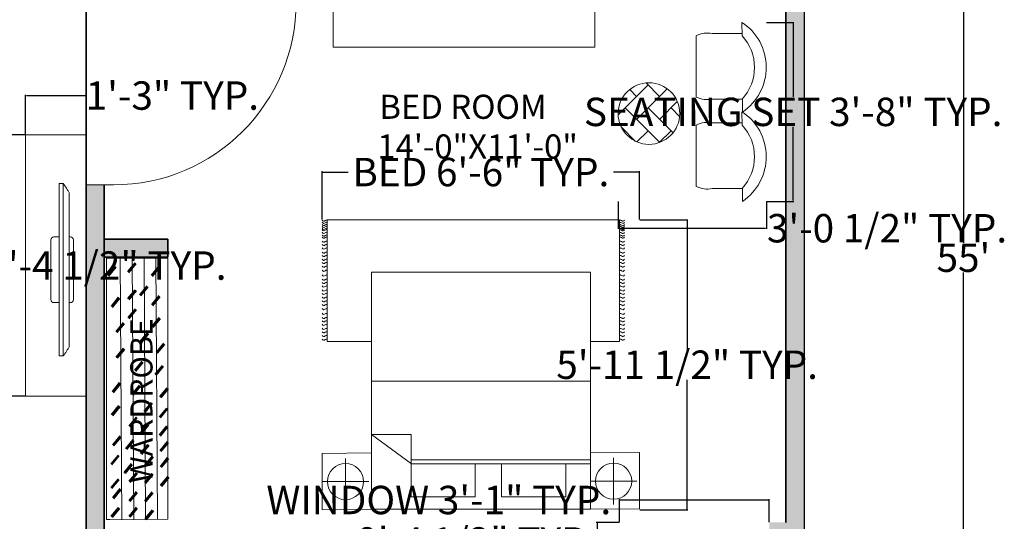
# Model space of a CAD drawing. Units: inches. Extents: x 0 to 4258, y 0 to 3769.
# Tile 25 of 30: x 3845 to 4088, y 3261 to 3385. Entities that reach past the tile are written whole.
import ezdxf

# ---------------------------------------------------------------- set-up
doc = ezdxf.new("R2010")
doc.units = ezdxf.units.IN
doc.header["$MEASUREMENT"] = 0
doc.layers.get('0').update_dxf_attribs({"color": 16})
for name, color, linetype, lineweight in [('A-ANNO-DIMS', 250, 'Continuous', 18), ('A-ANNO-TEXT', 250, 'Continuous', 18), ('A-AREA-IDEN', 250, 'Continuous', 18), ('A-CASE', 150, 'Continuous', 18), ('A-CASE-PATT', 251, 'Continuous', 13), ('A-EQPM', 8, 'Continuous', 18), ('A-WALL-PATT', 16, 'Continuous', 13), ('C-PROP', 150, 'Continuous', 25), ('doors', 250, 'Continuous', 18), ('furniture', 13, 'Continuous', 18), ('walls', 251, 'Continuous', 35)]:
    doc.layers.add(name, color=color, linetype=linetype, lineweight=lineweight)
doc.styles.get("Standard").update_dxf_attribs({"font": 'arial.ttf'})
doc.dimstyles.get("Standard").update_dxf_attribs({"dimtxt": 7, "dimasz": 0.18, "dimexe": 0.18, "dimexo": 0.0625, "dimgap": 0.09, "dimtad": 0, "dimtih": 1, "dimtoh": 1, "dimzin": 0, "dimdsep": 46, "dimlunit": 3, "dimtxsty": 'Standard', "dimcen": 0.09, "dimadec": 0, "dimazin": 0, "dimtfac": 1, "dimtofl": 0, "dimtmove": 0, "dimatfit": 3, "dimfxl": 1, "dimtolj": 1, "dimtzin": 0, "dimarcsym": 0})

# ---------------------------------------------------------------- blocks, each defined once
blk = doc.blocks.new('PLASMA-LARGE')
at = {"layer": 'furniture'}
for p, q in [((-7.26, 0), (7.26, 0)), ((-18.61, -1), (18.61, -1)), ((-8, -1), (-8, -0.74)), ((8, -1), (8, -0.74)), ((-21, -2.5), (21, -2.5)), ((-21, -2.5), (-21, -3.5)), ((-21, -3.5), (21, -3.5)), ((-8, -3.5), (-8, -4.76)), ((8, -3.5), (8, -4.76)), ((21, -2.5), (21, -3.5)), ((-7.26, -5.5), (7.26, -5.5))]:
    blk.add_line(p, q, dxfattribs=at)
for centre, radius, start, end in [((-7.26, -0.74), 0.744, 90, 180), ((7.26, -0.74), 0.744, 0, 90), ((-13.97, -11.05), 11.07, 114.7602, 129.4175), ((13.97, -11.05), 11.07, 50.5825, 65.2398), ((-7.26, -4.76), 0.744, 180, 270), ((7.26, -4.76), 0.744, 270, 0)]:
    blk.add_arc(centre, radius, start, end, dxfattribs=at)
blk = doc.blocks.new('CARPET')
at = {"layer": 'furniture'}
for p, q in [((-51.53, -98.11), (-51.53, -55.12)), ((-51.53, -55.12), (-41.27, -55.12)), ((36, -55.12), (51.55, -55.12)), ((51.55, -55.12), (51.55, -98.11)), ((51.55, -98.11), (-51.53, -98.11))]:
    blk.add_line(p, q, dxfattribs=at)
for points, knots in [([(-53.37, -55.99), (-53.22, -55.8), (-52.9, -55.41), (-52.34, -55.8), (-51.89, -56.08), (-51.65, -55.91), (-51.53, -55.83)], [0, 0, 0, 0, 0.653278, 1.290138, 1.740457, 2.114451, 2.114451, 2.114451, 2.114451]), ([(53.37, -55.99), (53.22, -55.8), (52.9, -55.41), (52.34, -55.8), (51.89, -56.08), (51.65, -55.91), (51.53, -55.83)], [0, 0, 0, 0, 0.653278, 1.290138, 1.740457, 2.114451, 2.114451, 2.114451, 2.114451]), ([(-53.37, -57.26), (-53.22, -57.07), (-52.9, -56.67), (-52.34, -57.07), (-51.89, -57.35), (-51.65, -57.17), (-51.53, -57.1)], [0, 0, 0, 0, 0.653278, 1.290138, 1.740457, 2.114451, 2.114451, 2.114451, 2.114451]), ([(-53.37, -58.59), (-53.22, -58.4), (-52.9, -58.01), (-52.34, -58.4), (-51.89, -58.68), (-51.65, -58.5), (-51.53, -58.43)], [0, 0, 0, 0, 0.653278, 1.290138, 1.740457, 2.114451, 2.114451, 2.114451, 2.114451]), ([(53.37, -57.26), (53.22, -57.07), (52.9, -56.67), (52.34, -57.07), (51.89, -57.35), (51.65, -57.17), (51.53, -57.1)], [0, 0, 0, 0, 0.653278, 1.290138, 1.740457, 2.114451, 2.114451, 2.114451, 2.114451]), ([(53.37, -58.59), (53.22, -58.4), (52.9, -58.01), (52.34, -58.4), (51.89, -58.68), (51.65, -58.5), (51.53, -58.43)], [0, 0, 0, 0, 0.653278, 1.290138, 1.740457, 2.114451, 2.114451, 2.114451, 2.114451]), ([(-53.37, -59.78), (-53.22, -59.58), (-52.9, -59.19), (-52.34, -59.58), (-51.89, -59.86), (-51.65, -59.69), (-51.53, -59.61)], [0, 0, 0, 0, 0.653278, 1.290138, 1.740457, 2.114451, 2.114451, 2.114451, 2.114451]), ([(-53.37, -61.22), (-53.22, -61.02), (-52.9, -60.63), (-52.34, -61.02), (-51.89, -61.3), (-51.65, -61.13), (-51.53, -61.05)], [0, 0, 0, 0, 0.653278, 1.290138, 1.740457, 2.114451, 2.114451, 2.114451, 2.114451]), ([(-53.37, -62.44), (-53.22, -62.25), (-52.9, -61.86), (-52.34, -62.25), (-51.89, -62.53), (-51.65, -62.36), (-51.53, -62.28)], [0, 0, 0, 0, 0.653278, 1.290138, 1.740457, 2.114451, 2.114451, 2.114451, 2.114451]), ([(53.37, -59.78), (53.22, -59.58), (52.9, -59.19), (52.34, -59.58), (51.89, -59.86), (51.65, -59.69), (51.53, -59.61)], [0, 0, 0, 0, 0.653278, 1.290138, 1.740457, 2.114451, 2.114451, 2.114451, 2.114451]), ([(53.37, -61.22), (53.22, -61.02), (52.9, -60.63), (52.34, -61.02), (51.89, -61.3), (51.65, -61.13), (51.53, -61.05)], [0, 0, 0, 0, 0.653278, 1.290138, 1.740457, 2.114451, 2.114451, 2.114451, 2.114451]), ([(53.37, -62.44), (53.22, -62.25), (52.9, -61.86), (52.34, -62.25), (51.89, -62.53), (51.65, -62.36), (51.53, -62.28)], [0, 0, 0, 0, 0.653278, 1.290138, 1.740457, 2.114451, 2.114451, 2.114451, 2.114451]), ([(-53.37, -63.63), (-53.22, -63.43), (-52.9, -63.04), (-52.34, -63.43), (-51.89, -63.72), (-51.65, -63.54), (-51.53, -63.46)], [0, 0, 0, 0, 0.653278, 1.290138, 1.740457, 2.114451, 2.114451, 2.114451, 2.114451]), ([(-53.37, -65.07), (-53.22, -64.87), (-52.9, -64.48), (-52.34, -64.87), (-51.89, -65.15), (-51.65, -64.98), (-51.53, -64.9)], [0, 0, 0, 0, 0.653278, 1.290138, 1.740457, 2.114451, 2.114451, 2.114451, 2.114451]), ([(53.37, -63.63), (53.22, -63.43), (52.9, -63.04), (52.34, -63.43), (51.89, -63.72), (51.65, -63.54), (51.53, -63.46)], [0, 0, 0, 0, 0.653278, 1.290138, 1.740457, 2.114451, 2.114451, 2.114451, 2.114451]), ([(53.37, -65.07), (53.22, -64.87), (52.9, -64.48), (52.34, -64.87), (51.89, -65.15), (51.65, -64.98), (51.53, -64.9)], [0, 0, 0, 0, 0.653278, 1.290138, 1.740457, 2.114451, 2.114451, 2.114451, 2.114451]), ([(-53.37, -66.76), (-53.22, -66.56), (-52.9, -66.17), (-52.34, -66.56), (-51.89, -66.84), (-51.65, -66.67), (-51.53, -66.59)], [0, 0, 0, 0, 0.653278, 1.290138, 1.740457, 2.114451, 2.114451, 2.114451, 2.114451]), ([(-53.37, -68.2), (-53.22, -68), (-52.9, -67.61), (-52.34, -68), (-51.89, -68.28), (-51.65, -68.11), (-51.53, -68.03)], [0, 0, 0, 0, 0.653278, 1.290138, 1.740457, 2.114451, 2.114451, 2.114451, 2.114451]), ([(-53.37, -69.53), (-53.22, -69.33), (-52.9, -68.94), (-52.34, -69.33), (-51.89, -69.61), (-51.65, -69.44), (-51.53, -69.36)], [0, 0, 0, 0, 0.653278, 1.290138, 1.740457, 2.114451, 2.114451, 2.114451, 2.114451]), ([(53.37, -66.76), (53.22, -66.56), (52.9, -66.17), (52.34, -66.56), (51.89, -66.84), (51.65, -66.67), (51.53, -66.59)], [0, 0, 0, 0, 0.653278, 1.290138, 1.740457, 2.114451, 2.114451, 2.114451, 2.114451]), ([(53.37, -68.2), (53.22, -68), (52.9, -67.61), (52.34, -68), (51.89, -68.28), (51.65, -68.11), (51.53, -68.03)], [0, 0, 0, 0, 0.653278, 1.290138, 1.740457, 2.114451, 2.114451, 2.114451, 2.114451]), ([(53.37, -69.53), (53.22, -69.33), (52.9, -68.94), (52.34, -69.33), (51.89, -69.61), (51.65, -69.44), (51.53, -69.36)], [0, 0, 0, 0, 0.653278, 1.290138, 1.740457, 2.114451, 2.114451, 2.114451, 2.114451]), ([(-53.37, -70.79), (-53.22, -70.6), (-52.9, -70.21), (-52.34, -70.6), (-51.89, -70.88), (-51.65, -70.7), (-51.53, -70.63)], [0, 0, 0, 0, 0.653278, 1.290138, 1.740457, 2.114451, 2.114451, 2.114451, 2.114451]), ([(-53.37, -72.12), (-53.22, -71.93), (-52.9, -71.54), (-52.34, -71.93), (-51.89, -72.21), (-51.65, -72.04), (-51.53, -71.96)], [0, 0, 0, 0, 0.653278, 1.290138, 1.740457, 2.114451, 2.114451, 2.114451, 2.114451]), ([(-53.37, -73.31), (-53.22, -73.11), (-52.9, -72.72), (-52.34, -73.11), (-51.89, -73.4), (-51.65, -73.22), (-51.53, -73.14)], [0, 0, 0, 0, 0.653278, 1.290138, 1.740457, 2.114451, 2.114451, 2.114451, 2.114451]), ([(53.37, -70.79), (53.22, -70.6), (52.9, -70.21), (52.34, -70.6), (51.89, -70.88), (51.65, -70.7), (51.53, -70.63)], [0, 0, 0, 0, 0.653278, 1.290138, 1.740457, 2.114451, 2.114451, 2.114451, 2.114451]), ([(53.37, -72.12), (53.22, -71.93), (52.9, -71.54), (52.34, -71.93), (51.89, -72.21), (51.65, -72.04), (51.53, -71.96)], [0, 0, 0, 0, 0.653278, 1.290138, 1.740457, 2.114451, 2.114451, 2.114451, 2.114451]), ([(53.37, -73.31), (53.22, -73.11), (52.9, -72.72), (52.34, -73.11), (51.89, -73.4), (51.65, -73.22), (51.53, -73.14)], [0, 0, 0, 0, 0.653278, 1.290138, 1.740457, 2.114451, 2.114451, 2.114451, 2.114451]), ([(-53.37, -74.75), (-53.22, -74.55), (-52.9, -74.16), (-52.34, -74.55), (-51.89, -74.83), (-51.65, -74.66), (-51.53, -74.58)], [0, 0, 0, 0, 0.653278, 1.290138, 1.740457, 2.114451, 2.114451, 2.114451, 2.114451]), ([(-53.37, -75.98), (-53.22, -75.78), (-52.9, -75.39), (-52.34, -75.78), (-51.89, -76.06), (-51.65, -75.89), (-51.53, -75.81)], [0, 0, 0, 0, 0.653278, 1.290138, 1.740457, 2.114451, 2.114451, 2.114451, 2.114451]), ([(53.37, -74.75), (53.22, -74.55), (52.9, -74.16), (52.34, -74.55), (51.89, -74.83), (51.65, -74.66), (51.53, -74.58)], [0, 0, 0, 0, 0.653278, 1.290138, 1.740457, 2.114451, 2.114451, 2.114451, 2.114451]), ([(53.37, -75.98), (53.22, -75.78), (52.9, -75.39), (52.34, -75.78), (51.89, -76.06), (51.65, -75.89), (51.53, -75.81)], [0, 0, 0, 0, 0.653278, 1.290138, 1.740457, 2.114451, 2.114451, 2.114451, 2.114451]), ([(-53.37, -77.16), (-53.22, -76.96), (-52.9, -76.57), (-52.34, -76.96), (-51.89, -77.25), (-51.65, -77.07), (-51.53, -76.99)], [0, 0, 0, 0, 0.653278, 1.290138, 1.740457, 2.114451, 2.114451, 2.114451, 2.114451]), ([(-53.37, -78.6), (-53.22, -78.4), (-52.9, -78.01), (-52.34, -78.4), (-51.89, -78.68), (-51.65, -78.51), (-51.53, -78.43)], [0, 0, 0, 0, 0.653278, 1.290138, 1.740457, 2.114451, 2.114451, 2.114451, 2.114451]), ([(-53.37, -80.29), (-53.22, -80.09), (-52.9, -79.7), (-52.34, -80.09), (-51.89, -80.37), (-51.65, -80.2), (-51.53, -80.12)], [0, 0, 0, 0, 0.653278, 1.290138, 1.740457, 2.114451, 2.114451, 2.114451, 2.114451]), ([(53.37, -77.16), (53.22, -76.96), (52.9, -76.57), (52.34, -76.96), (51.89, -77.25), (51.65, -77.07), (51.53, -76.99)], [0, 0, 0, 0, 0.653278, 1.290138, 1.740457, 2.114451, 2.114451, 2.114451, 2.114451]), ([(53.37, -78.6), (53.22, -78.4), (52.9, -78.01), (52.34, -78.4), (51.89, -78.68), (51.65, -78.51), (51.53, -78.43)], [0, 0, 0, 0, 0.653278, 1.290138, 1.740457, 2.114451, 2.114451, 2.114451, 2.114451]), ([(53.37, -80.29), (53.22, -80.09), (52.9, -79.7), (52.34, -80.09), (51.89, -80.37), (51.65, -80.2), (51.53, -80.12)], [0, 0, 0, 0, 0.653278, 1.290138, 1.740457, 2.114451, 2.114451, 2.114451, 2.114451]), ([(-53.37, -81.73), (-53.22, -81.53), (-52.9, -81.14), (-52.34, -81.53), (-51.89, -81.81), (-51.65, -81.64), (-51.53, -81.56)], [0, 0, 0, 0, 0.653278, 1.290138, 1.740457, 2.114451, 2.114451, 2.114451, 2.114451]), ([(-53.37, -83.06), (-53.22, -82.86), (-52.9, -82.47), (-52.34, -82.86), (-51.89, -83.14), (-51.65, -82.97), (-51.53, -82.89)], [0, 0, 0, 0, 0.653278, 1.290138, 1.740457, 2.114451, 2.114451, 2.114451, 2.114451]), ([(53.37, -81.73), (53.22, -81.53), (52.9, -81.14), (52.34, -81.53), (51.89, -81.81), (51.65, -81.64), (51.53, -81.56)], [0, 0, 0, 0, 0.653278, 1.290138, 1.740457, 2.114451, 2.114451, 2.114451, 2.114451]), ([(53.37, -83.06), (53.22, -82.86), (52.9, -82.47), (52.34, -82.86), (51.89, -83.14), (51.65, -82.97), (51.53, -82.89)], [0, 0, 0, 0, 0.653278, 1.290138, 1.740457, 2.114451, 2.114451, 2.114451, 2.114451]), ([(-53.37, -84.18), (-53.22, -83.99), (-52.9, -83.6), (-52.34, -83.99), (-51.89, -84.27), (-51.65, -84.09), (-51.53, -84.02)], [0, 0, 0, 0, 0.653278, 1.290138, 1.740457, 2.114451, 2.114451, 2.114451, 2.114451]), ([(-53.37, -85.51), (-53.22, -85.32), (-52.9, -84.93), (-52.34, -85.32), (-51.89, -85.6), (-51.65, -85.42), (-51.53, -85.35)], [0, 0, 0, 0, 0.653278, 1.290138, 1.740457, 2.114451, 2.114451, 2.114451, 2.114451]), ([(-53.37, -86.7), (-53.22, -86.5), (-52.9, -86.11), (-52.34, -86.5), (-51.89, -86.78), (-51.65, -86.61), (-51.53, -86.53)], [0, 0, 0, 0, 0.653278, 1.290138, 1.740457, 2.114451, 2.114451, 2.114451, 2.114451]), ([(53.37, -84.18), (53.22, -83.99), (52.9, -83.6), (52.34, -83.99), (51.89, -84.27), (51.65, -84.09), (51.53, -84.02)], [0, 0, 0, 0, 0.653278, 1.290138, 1.740457, 2.114451, 2.114451, 2.114451, 2.114451]), ([(53.37, -85.51), (53.22, -85.32), (52.9, -84.93), (52.34, -85.32), (51.89, -85.6), (51.65, -85.42), (51.53, -85.35)], [0, 0, 0, 0, 0.653278, 1.290138, 1.740457, 2.114451, 2.114451, 2.114451, 2.114451]), ([(53.37, -86.7), (53.22, -86.5), (52.9, -86.11), (52.34, -86.5), (51.89, -86.78), (51.65, -86.61), (51.53, -86.53)], [0, 0, 0, 0, 0.653278, 1.290138, 1.740457, 2.114451, 2.114451, 2.114451, 2.114451]), ([(-53.37, -88.14), (-53.22, -87.94), (-52.9, -87.55), (-52.34, -87.94), (-51.89, -88.22), (-51.65, -88.05), (-51.53, -87.97)], [0, 0, 0, 0, 0.653278, 1.290138, 1.740457, 2.114451, 2.114451, 2.114451, 2.114451]), ([(-53.37, -89.36), (-53.22, -89.17), (-52.9, -88.78), (-52.34, -89.17), (-51.89, -89.45), (-51.65, -89.28), (-51.53, -89.2)], [0, 0, 0, 0, 0.653278, 1.290138, 1.740457, 2.114451, 2.114451, 2.114451, 2.114451]), ([(-53.37, -90.55), (-53.22, -90.35), (-52.9, -89.96), (-52.34, -90.35), (-51.89, -90.64), (-51.65, -90.46), (-51.53, -90.38)], [0, 0, 0, 0, 0.653278, 1.290138, 1.740457, 2.114451, 2.114451, 2.114451, 2.114451]), ([(53.37, -88.14), (53.22, -87.94), (52.9, -87.55), (52.34, -87.94), (51.89, -88.22), (51.65, -88.05), (51.53, -87.97)], [0, 0, 0, 0, 0.653278, 1.290138, 1.740457, 2.114451, 2.114451, 2.114451, 2.114451]), ([(53.37, -89.36), (53.22, -89.17), (52.9, -88.78), (52.34, -89.17), (51.89, -89.45), (51.65, -89.28), (51.53, -89.2)], [0, 0, 0, 0, 0.653278, 1.290138, 1.740457, 2.114451, 2.114451, 2.114451, 2.114451]), ([(53.37, -90.55), (53.22, -90.35), (52.9, -89.96), (52.34, -90.35), (51.9, -90.63), (51.66, -90.47), (51.55, -90.4)], [0, 0, 0, 0, 0.653278, 1.290138, 1.740457, 2.0926, 2.0926, 2.0926, 2.0926]), ([(-53.37, -91.99), (-53.22, -91.79), (-52.9, -91.4), (-52.34, -91.79), (-51.89, -92.07), (-51.65, -91.9), (-51.53, -91.82)], [0, 0, 0, 0, 0.653278, 1.290138, 1.740457, 2.114451, 2.114451, 2.114451, 2.114451]), ([(-53.37, -92.69), (-53.22, -92.48), (-52.9, -92.08), (-52.35, -92.49), (-51.89, -92.77), (-51.65, -92.6), (-51.53, -92.52)], [0, 0, 0, 0, 0.663904, 1.307406, 1.757725, 2.131719, 2.131719, 2.131719, 2.131719]), ([(-53.37, -93.61), (-53.22, -93.42), (-52.9, -93.03), (-52.34, -93.42), (-51.89, -93.7), (-51.65, -93.52), (-51.53, -93.45)], [0, 0, 0, 0, 0.653278, 1.290138, 1.740457, 2.114451, 2.114451, 2.114451, 2.114451]), ([(53.37, -91.99), (53.22, -91.79), (52.9, -91.4), (52.34, -91.79), (51.9, -92.07), (51.66, -91.91), (51.55, -91.83)], [0, 0, 0, 0, 0.653278, 1.290138, 1.740457, 2.0926, 2.0926, 2.0926, 2.0926]), ([(53.37, -92.69), (53.22, -92.49), (52.9, -92.09), (52.34, -92.49), (51.9, -92.77), (51.66, -92.61), (51.55, -92.53)], [0, 0, 0, 0, 0.656792, 1.295826, 1.746145, 2.098292, 2.098292, 2.098292, 2.098292]), ([(53.37, -93.66), (53.22, -93.46), (52.9, -93.07), (52.34, -93.46), (51.9, -93.74), (51.66, -93.58), (51.55, -93.5)], [0, 0, 0, 0, 0.653278, 1.290138, 1.740457, 2.0926, 2.0926, 2.0926, 2.0926]), ([(-53.37, -94.55), (-53.22, -94.35), (-52.9, -93.96), (-52.34, -94.35), (-51.89, -94.63), (-51.65, -94.46), (-51.53, -94.38)], [0, 0, 0, 0, 0.653278, 1.290138, 1.740457, 2.114451, 2.114451, 2.114451, 2.114451]), ([(-53.37, -95.05), (-53.22, -94.85), (-52.9, -94.46), (-52.34, -94.85), (-51.89, -95.14), (-51.65, -94.96), (-51.53, -94.88)], [0, 0, 0, 0, 0.653278, 1.290138, 1.740457, 2.114451, 2.114451, 2.114451, 2.114451]), ([(-53.37, -95.73), (-53.22, -95.54), (-52.9, -95.15), (-52.34, -95.54), (-51.89, -95.82), (-51.65, -95.65), (-51.53, -95.57)], [0, 0, 0, 0, 0.653278, 1.290138, 1.740457, 2.114451, 2.114451, 2.114451, 2.114451]), ([(-53.37, -96.38), (-53.22, -96.18), (-52.9, -95.79), (-52.34, -96.18), (-51.89, -96.47), (-51.65, -96.29), (-51.53, -96.21)], [0, 0, 0, 0, 0.653278, 1.290138, 1.740457, 2.114451, 2.114451, 2.114451, 2.114451]), ([(-53.37, -97.17), (-53.22, -96.98), (-52.9, -96.59), (-52.34, -96.98), (-51.89, -97.26), (-51.65, -97.08), (-51.53, -97.01)], [0, 0, 0, 0, 0.653278, 1.290138, 1.740457, 2.114451, 2.114451, 2.114451, 2.114451]), ([(53.37, -95.78), (53.22, -95.58), (52.9, -95.19), (52.34, -95.58), (51.89, -95.86), (51.65, -95.69), (51.53, -95.61)], [0, 0, 0, 0, 0.653278, 1.290138, 1.740457, 2.114451, 2.114451, 2.114451, 2.114451]), ([(53.37, -96.43), (53.22, -96.23), (52.9, -95.84), (52.34, -96.23), (51.89, -96.51), (51.65, -96.34), (51.53, -96.26)], [0, 0, 0, 0, 0.653278, 1.290138, 1.740457, 2.114451, 2.114451, 2.114451, 2.114451]), ([(53.37, -97.22), (53.22, -97.02), (52.9, -96.63), (52.34, -97.02), (51.89, -97.3), (51.65, -97.13), (51.53, -97.05)], [0, 0, 0, 0, 0.653278, 1.290138, 1.740457, 2.114451, 2.114451, 2.114451, 2.114451]), ([(53.37, -94.59), (53.22, -94.4), (52.9, -94.01), (52.34, -94.4), (51.9, -94.68), (51.66, -94.51), (51.55, -94.44)], [0, 0, 0, 0, 0.653278, 1.290138, 1.740457, 2.0926, 2.0926, 2.0926, 2.0926]), ([(53.37, -95.1), (53.22, -94.9), (52.9, -94.51), (52.34, -94.9), (51.9, -95.18), (51.66, -95.02), (51.55, -94.94)], [0, 0, 0, 0, 0.653278, 1.290138, 1.740457, 2.0926, 2.0926, 2.0926, 2.0926]), ([(-53.37, -97.99), (-53.22, -97.79), (-52.9, -97.4), (-52.34, -97.79), (-51.89, -98.08), (-51.65, -97.9), (-51.53, -97.82)], [0, 0, 0, 0, 0.653278, 1.290138, 1.740457, 2.114451, 2.114451, 2.114451, 2.114451]), ([(53.37, -97.99), (53.22, -97.79), (52.9, -97.4), (52.34, -97.79), (51.89, -98.08), (51.65, -97.9), (51.53, -97.82)], [0, 0, 0, 0, 0.653278, 1.290138, 1.740457, 2.114451, 2.114451, 2.114451, 2.114451])]:
    blk.add_open_spline(points, degree=3, knots=knots, dxfattribs=at)
blk = doc.blocks.new('A$C58D270C6')
at = {"layer": 'furniture'}
for p, q in [((9.09, 124.13), (9.09, 108.87)), ((1.46, 116.5), (16.73, 116.5)), ((14.97, 94.84), (24.62, 107.92)), ((24.62, 94.93), (24.62, 107.92)), ((42.08, 108), (42.08, 36)), ((14.97, 94.93), (24.62, 94.93)), ((14.97, 94.84), (14.97, 36)), ((16.22, 94.93), (16.22, 36)), ((9.25, 36), (9.25, 20.74)), ((1.62, 28.37), (16.88, 28.37))]:
    blk.add_line(p, q, dxfattribs=at)
for points in [[(18.5, 108), (18.34, 124.13), (-0.16, 124.13), (0, 108)], [(0, 108), (77.91, 108), (77.91, 36), (0, 36)], [(4.09, 94.93), (14.97, 94.93), (14.97, 73.83), (4.09, 73.83)], [(4.09, 65.23), (14.97, 65.23), (14.97, 44.13), (4.09, 44.13)], [(18.65, 19.87), (18.5, 36), (0, 36), (0.16, 19.87)]]:
    blk.add_lwpolyline(points, close=True, dxfattribs=at)
for centre in [(9.09, 116.5), (9.25, 28.37)]:
    blk.add_circle(centre, 5.95, dxfattribs=at)
at = {"layer": 'furniture', "xscale": 0.9312884925094044, "yscale": 0.9312884925094044, "zscale": 0.9312884925094044, "rotation": 90}
blk.add_blockref('CARPET', (3.79, 74.47), dxfattribs=at)
blk = doc.blocks.new('*U23')
for p, q in [((0, 0), (0, -6)), ((40, 0), (40, -6))]:
    blk.add_line(p, q)
blk.add_lwpolyline([(0, 0), (0, 40), (1.75, 40), (1.75, 0)], close=True)
blk.add_arc((0, 0), 40, 0, 90)
blk = doc.blocks.new('*D26')
at = {"layer": 'A-ANNO-DIMS', "color": 0, "lineweight": -2, "transparency": 16777216}
for p, q in [((4077.41, 3656.79), (4078.27, 3656.79)), ((4078.09, 3656.61), (4078.09, 3329.69)), ((4078.09, 2995.47), (4078.09, 3322.39)), ((4077.41, 2995.29), (4078.27, 2995.29))]:
    blk.add_line(p, q, dxfattribs=at)
at = {"layer": 'A-ANNO-DIMS', "color": 0, "transparency": 16777216}
for points in [[(4078.06, 3656.61), (4078.12, 3656.61), (4078.09, 3656.79)], [(4078.06, 2995.47), (4078.12, 2995.47), (4078.09, 2995.29)]]:
    blk.add_solid(points, dxfattribs=at)
at = {"layer": 'Defpoints', "color": 0, "transparency": 16777216}
for p in [(4077.35, 3656.79), (4077.35, 2995.29), (4078.09, 2995.29)]:
    blk.add_point(p, dxfattribs=at)
at = {"layer": 'A-ANNO-DIMS', "color": 0, "transparency": 16777216, "insert": (4078.09, 3326.04), "char_height": 7, "attachment_point": 5}
blk.add_mtext("\\A1;55'", dxfattribs=at)
blk = doc.blocks.new('SEATING-TWO-CHAIRS-AND-TABLE')
h = blk.add_hatch()
h.set_pattern_fill('AR-HBONE', color=256, angle=90)
h.set_pattern_definition([(135, (3403.542, -4056.0025), (-5.6568542, 3e-16), [12, -4]), (225, (3400.7137, -4053.174), (-5.6568542, 8e-16), [12, -4])])
h.paths.add_polyline_path([(7.59, 14.04, 1), (7.59, 29.23, 1)])
for p, q in [((30.53, 40.83), (30.5, 44.11)), ((23.18, 41.34), (30.53, 41.34)), ((19.25, 25.7), (19.25, 40.83)), ((23.18, 25.19), (30.53, 25.19)), ((30.63, 22.02), (30.63, 25.19)), ((30.53, 18.81), (30.5, 22.09)), ((19.25, 3.68), (19.25, 18.81)), ((23.18, 19.32), (30.53, 19.32)), ((23.18, 3.17), (30.53, 3.17)), ((30.63, 0), (30.63, 3.17))]:
    blk.add_line(p, q)
blk.add_circle((7.59, 21.64), 7.59)
for centre, radius, start, end in [((23.25, 33.02), 13.25, 303.8239, 56.829), ((21.94, 35.53), 5.94, 77.9198, 116.8624), ((22.13, 33.01), 11.48, 317.0375, 42.9625), ((21.94, 31), 5.94, 243.1376, 282.0802), ((23.25, 11.01), 13.25, 303.8239, 56.829), ((21.94, 13.51), 5.94, 77.9198, 116.8624), ((22.13, 10.99), 11.48, 317.0375, 42.9625), ((21.94, 8.98), 5.94, 243.1376, 282.0802)]:
    blk.add_arc(centre, radius, start, end)
blk = doc.blocks.new('TV-CONSOLE-CABINET')
for p, q in [((0, 0), (0, 64.44)), ((0, 64.44), (14.9, 64.44)), ((14.9, 0), (0, 0))]:
    blk.add_line(p, q)
blk = doc.blocks.new('*D38')
at = {"layer": 'A-ANNO-DIMS', "color": 0, "lineweight": -2, "transparency": 16777216}
for p, q in [((3846.84, 3356.33), (3837.06, 3356.33)), ((3837.24, 3356.15), (3837.24, 3327.83)), ((3837.24, 3292.07), (3837.24, 3320.4)), ((3846.84, 3291.89), (3837.06, 3291.89))]:
    blk.add_line(p, q, dxfattribs=at)
at = {"layer": 'A-ANNO-DIMS', "color": 0, "transparency": 16777216}
for points in [[(3837.21, 3356.15), (3837.27, 3356.15), (3837.24, 3356.33)], [(3837.21, 3292.07), (3837.27, 3292.07), (3837.24, 3291.89)]]:
    blk.add_solid(points, dxfattribs=at)
at = {"layer": 'Defpoints', "color": 0, "transparency": 16777216}
for p in [(3837.24, 3356.33), (3846.91, 3356.33), (3846.91, 3291.89)]:
    blk.add_point(p, dxfattribs=at)
at = {"layer": 'A-ANNO-DIMS', "color": 0, "transparency": 16777216, "insert": (3837.24, 3324.11), "char_height": 7, "attachment_point": 5}
blk.add_mtext('\\A1;TV CONSOLE 5\'-4 1/2" TYP.', dxfattribs=at)
blk = doc.blocks.new('*D39')
at = {"layer": 'A-ANNO-DIMS', "color": 0, "lineweight": -2, "transparency": 16777216}
for p, q in [((3846.91, 3356.4), (3846.91, 3366.18)), ((3847.09, 3366), (3861.62, 3366)), ((3861.8, 3356.4), (3861.8, 3366.18)), ((3861.8, 3366), (3861.98, 3366))]:
    blk.add_line(p, q, dxfattribs=at)
at = {"layer": 'A-ANNO-DIMS', "color": 0, "transparency": 16777216}
for points in [[(3847.09, 3366.03), (3847.09, 3365.97), (3846.91, 3366)], [(3861.62, 3366.03), (3861.62, 3365.97), (3861.8, 3366)]]:
    blk.add_solid(points, dxfattribs=at)
at = {"layer": 'Defpoints', "color": 0, "transparency": 16777216}
for p in [(3861.8, 3366), (3846.91, 3356.33), (3861.8, 3356.33)]:
    blk.add_point(p, dxfattribs=at)
at = {"layer": 'A-ANNO-DIMS', "color": 0, "transparency": 16777216, "insert": (3883.08, 3366), "char_height": 7, "attachment_point": 5}
blk.add_mtext('\\A1;1\'-3" TYP.', dxfattribs=at)
blk = doc.blocks.new('*D48')
at = {"layer": 'A-ANNO-DIMS', "color": 0, "lineweight": -2, "transparency": 16777216}
for p, q in [((3920, 3335.47), (3920, 3347.33)), ((3920.18, 3347.15), (3926.44, 3347.15)), ((3998.05, 3347.15), (3991.8, 3347.15)), ((3998.23, 3335.47), (3998.23, 3347.33))]:
    blk.add_line(p, q, dxfattribs=at)
at = {"layer": 'A-ANNO-DIMS', "color": 0, "transparency": 16777216}
for points in [[(3920.18, 3347.18), (3920.18, 3347.12), (3920, 3347.15)], [(3998.05, 3347.18), (3998.05, 3347.12), (3998.23, 3347.15)]]:
    blk.add_solid(points, dxfattribs=at)
at = {"layer": 'Defpoints', "color": 0, "transparency": 16777216}
for p in [(3920, 3347.15), (3920, 3335.41), (3998.23, 3335.41)]:
    blk.add_point(p, dxfattribs=at)
at = {"layer": 'A-ANNO-DIMS', "color": 0, "transparency": 16777216, "insert": (3959.12, 3347.15), "char_height": 7, "attachment_point": 5}
blk.add_mtext('\\A1;BED 6\'-6" TYP.', dxfattribs=at)
blk = doc.blocks.new('*D49')
at = {"layer": 'A-ANNO-DIMS', "color": 0, "lineweight": -2, "transparency": 16777216}
for p, q in [((3998.3, 3335.41), (4010.15, 3335.41)), ((4009.97, 3335.23), (4009.97, 3303.38)), ((4009.97, 3264.11), (4009.97, 3295.96)), ((3998.3, 3263.93), (4010.15, 3263.93))]:
    blk.add_line(p, q, dxfattribs=at)
at = {"layer": 'A-ANNO-DIMS', "color": 0, "transparency": 16777216}
for points in [[(4009.94, 3335.23), (4010, 3335.23), (4009.97, 3335.41)], [(4009.94, 3264.11), (4010, 3264.11), (4009.97, 3263.93)]]:
    blk.add_solid(points, dxfattribs=at)
at = {"layer": 'Defpoints', "color": 0, "transparency": 16777216}
for p in [(3998.23, 3335.41), (4009.97, 3335.41), (3998.23, 3263.93)]:
    blk.add_point(p, dxfattribs=at)
at = {"layer": 'A-ANNO-DIMS', "color": 0, "transparency": 16777216, "insert": (4009.97, 3299.67), "char_height": 7, "attachment_point": 5}
blk.add_mtext('\\A1;5\'-11 1/2" TYP.', dxfattribs=at)
blk = doc.blocks.new('*D56')
at = {"layer": 'A-ANNO-DIMS', "color": 0, "lineweight": -2, "transparency": 16777216}
for p, q in [((4029.56, 3384.04), (4036.29, 3384.04)), ((4036.11, 3383.86), (4036.11, 3365.7)), ((4036.11, 3340.11), (4036.11, 3358.27)), ((4029.56, 3339.93), (4036.29, 3339.93))]:
    blk.add_line(p, q, dxfattribs=at)
at = {"layer": 'A-ANNO-DIMS', "color": 0, "transparency": 16777216}
for points in [[(4036.08, 3383.86), (4036.14, 3383.86), (4036.11, 3384.04)], [(4036.08, 3340.11), (4036.14, 3340.11), (4036.11, 3339.93)]]:
    blk.add_solid(points, dxfattribs=at)
at = {"layer": 'Defpoints', "color": 0, "transparency": 16777216}
for p in [(4029.5, 3384.04), (4036.11, 3384.04), (4029.5, 3339.93)]:
    blk.add_point(p, dxfattribs=at)
at = {"layer": 'A-ANNO-DIMS', "color": 0, "transparency": 16777216, "insert": (4036.11, 3361.98), "char_height": 7, "attachment_point": 5}
blk.add_mtext('\\A1;SEATING SET 3\'-8" TYP.', dxfattribs=at)
blk = doc.blocks.new('*D57')
at = {"layer": 'A-ANNO-DIMS', "color": 0, "lineweight": -2, "transparency": 16777216}
for p, q in [((3992.97, 3339.87), (3992.97, 3333.13)), ((4029.5, 3339.87), (4029.5, 3333.13)), ((3993.15, 3333.31), (4029.32, 3333.31)), ((4029.5, 3333.31), (4029.68, 3333.31))]:
    blk.add_line(p, q, dxfattribs=at)
at = {"layer": 'A-ANNO-DIMS', "color": 0, "transparency": 16777216}
for points in [[(3993.15, 3333.34), (3993.15, 3333.28), (3992.97, 3333.31)], [(4029.32, 3333.34), (4029.32, 3333.28), (4029.5, 3333.31)]]:
    blk.add_solid(points, dxfattribs=at)
at = {"layer": 'Defpoints', "color": 0, "transparency": 16777216}
for p in [(3992.97, 3339.93), (4029.5, 3339.93), (4029.5, 3333.31)]:
    blk.add_point(p, dxfattribs=at)
at = {"layer": 'A-ANNO-DIMS', "color": 0, "transparency": 16777216, "insert": (4059.25, 3333.31), "char_height": 7, "attachment_point": 5}
blk.add_mtext('\\A1;3\'-0 1/2" TYP.', dxfattribs=at)
blk = doc.blocks.new('*D58')
at = {"layer": 'A-ANNO-DIMS', "color": 0, "lineweight": -2, "transparency": 16777216}
for p, q in [((3993.31, 3266.33), (3993.13, 3266.33)), ((3993.31, 3260.86), (3993.31, 3266.51)), ((4030.03, 3266.33), (3993.49, 3266.33)), ((4030.21, 3260.86), (4030.21, 3266.51))]:
    blk.add_line(p, q, dxfattribs=at)
at = {"layer": 'A-ANNO-DIMS', "color": 0, "transparency": 16777216}
for points in [[(3993.49, 3266.36), (3993.49, 3266.3), (3993.31, 3266.33)], [(4030.03, 3266.36), (4030.03, 3266.3), (4030.21, 3266.33)]]:
    blk.add_solid(points, dxfattribs=at)
at = {"layer": 'Defpoints', "color": 0, "transparency": 16777216}
for p in [(3993.31, 3266.33), (3993.31, 3260.79), (4030.21, 3260.79)]:
    blk.add_point(p, dxfattribs=at)
at = {"layer": 'A-ANNO-DIMS', "color": 0, "transparency": 16777216, "insert": (3948.75, 3266.33), "char_height": 7, "attachment_point": 5}
blk.add_mtext('\\A1;WINDOW 3\'-1" TYP.', dxfattribs=at)
blk = doc.blocks.new('*D59')
at = {"layer": 'A-ANNO-DIMS', "color": 0, "lineweight": -2, "transparency": 16777216}
for p, q in [((3993.24, 3260.79), (3987.59, 3260.79)), ((3987.77, 3260.61), (3987.77, 3256.47)), ((3993.24, 3256.29), (3987.59, 3256.29)), ((3987.77, 3256.11), (3987.59, 3256.11)), ((3987.77, 3256.29), (3987.77, 3256.11))]:
    blk.add_line(p, q, dxfattribs=at)
at = {"layer": 'A-ANNO-DIMS', "color": 0, "transparency": 16777216}
for points in [[(3987.74, 3260.61), (3987.8, 3260.61), (3987.77, 3260.79)], [(3987.74, 3256.47), (3987.8, 3256.47), (3987.77, 3256.29)]]:
    blk.add_solid(points, dxfattribs=at)
at = {"layer": 'Defpoints', "color": 0, "transparency": 16777216}
for p in [(3993.31, 3260.79), (3987.77, 3256.29), (3993.31, 3256.29)]:
    blk.add_point(p, dxfattribs=at)
at = {"layer": 'A-ANNO-DIMS', "color": 0, "transparency": 16777216, "insert": (3958.01, 3256.11), "char_height": 7, "attachment_point": 5}
blk.add_mtext('\\A1;0\'-4 1/2" TYP.', dxfattribs=at)

msp = doc.modelspace()

# ---------------------------------------------------------------- hatches: boundary and pattern name
at = {"layer": 'A-CASE-PATT'}
h = msp.add_hatch(dxfattribs=at)
h.set_pattern_fill('ANSI31', color=256, scale=0.92773417, angle=5.4670054, style=0)
h.paths.add_polyline_path([(3878.558, 3263.559), (3876.754, 3261.373), (3876.307, 3261.742), (3878.111, 3263.928)])
h.paths.add_polyline_path([(3882.282, 3271.824), (3880.478, 3269.638), (3880.031, 3270.007), (3881.835, 3272.193)], flags=0)
h.paths.add_polyline_path([(3878.393, 3268.004), (3876.589, 3265.818), (3876.141, 3266.187), (3877.945, 3268.373)], flags=0)
h.paths.add_polyline_path([(3874.571, 3264.185), (3872.767, 3261.999), (3872.32, 3262.368), (3874.124, 3264.554)], flags=0)
h.paths.add_polyline_path([(3882.222, 3276.493), (3880.418, 3274.307), (3879.971, 3274.676), (3881.775, 3276.862)], flags=0)
h.paths.add_polyline_path([(3878.446, 3272.541), (3876.642, 3270.355), (3876.195, 3270.724), (3877.999, 3272.91)], flags=0)
h.paths.add_polyline_path([(3874.548, 3268.098), (3872.744, 3265.912), (3872.297, 3266.281), (3874.101, 3268.467)], flags=0)
h.paths.add_polyline_path([(3870.138, 3264.187), (3868.334, 3262.001), (3867.886, 3262.371), (3869.691, 3264.556)], flags=0)
h.paths.add_polyline_path([(3882.199, 3280.389), (3880.395, 3278.203), (3879.947, 3278.573), (3881.752, 3280.758)], flags=0)
h.paths.add_polyline_path([(3878.555, 3276.841), (3876.751, 3274.655), (3876.303, 3275.024), (3878.107, 3277.21)], flags=0)
h.paths.add_polyline_path([(3874.521, 3272.798), (3872.717, 3270.612), (3872.269, 3270.982), (3874.073, 3273.167)], flags=0)
h.paths.add_polyline_path([(3870.465, 3268.832), (3868.661, 3266.646), (3868.213, 3267.015), (3870.017, 3269.201)], flags=0)
h.paths.add_polyline_path([(3882.04, 3284.231), (3880.236, 3282.045), (3879.788, 3282.414), (3881.592, 3284.6)], flags=0)
h.paths.add_polyline_path([(3877.407, 3279.694), (3875.602, 3277.508), (3875.155, 3277.877), (3876.959, 3280.063)], flags=0)
h.paths.add_polyline_path([(3873.334, 3274.981), (3871.53, 3272.796), (3871.083, 3273.165), (3872.887, 3275.351)], flags=0)
h.paths.add_polyline_path([(3870.004, 3271.301), (3868.2, 3269.115), (3867.842, 3269.41), (3869.646, 3271.596)], flags=0)
h.paths.add_polyline_path([(3881.963, 3288.746), (3880.159, 3286.56), (3879.802, 3286.855), (3881.606, 3289.041)], flags=0)
h.paths.add_polyline_path([(3877.377, 3284.708), (3875.573, 3282.522), (3875.126, 3282.891), (3876.93, 3285.077)], flags=0)
h.paths.add_polyline_path([(3873.721, 3280.914), (3871.917, 3278.728), (3871.47, 3279.097), (3873.274, 3281.283)], flags=0)
h.paths.add_polyline_path([(3870.026, 3277.134), (3868.222, 3274.948), (3867.865, 3275.243), (3869.669, 3277.429)], flags=0)
h.paths.add_polyline_path([(3882.11, 3293.679), (3880.306, 3291.493), (3879.859, 3291.862), (3881.663, 3294.048)], flags=0)
h.paths.add_polyline_path([(3878.28, 3290.033), (3876.476, 3287.847), (3876.029, 3288.216), (3877.833, 3290.402)], flags=0)
h.paths.add_polyline_path([(3874.44, 3286.521), (3872.636, 3284.335), (3872.278, 3284.63), (3874.082, 3286.816)], flags=0)
h.paths.add_polyline_path([(3870.581, 3281.756), (3868.777, 3279.57), (3868.33, 3279.939), (3870.134, 3282.125)], flags=0)
h.paths.add_polyline_path([(3881.003, 3299.141), (3879.199, 3296.955), (3878.752, 3297.324), (3880.556, 3299.51)], flags=0)
h.paths.add_polyline_path([(3875.3, 3294.231), (3873.496, 3292.045), (3873.048, 3292.414), (3874.853, 3294.6)], flags=0)
h.paths.add_polyline_path([(3870.269, 3289.236), (3868.465, 3287.05), (3868.017, 3287.419), (3869.821, 3289.605)], flags=0)
h.paths.add_polyline_path([(3881.239, 3304.645), (3879.435, 3302.46), (3878.988, 3302.829), (3880.792, 3305.015)], flags=0)
h.paths.add_polyline_path([(3875.937, 3300.185), (3874.133, 3297.999), (3873.685, 3298.368), (3875.489, 3300.554)], flags=0)
h.paths.add_polyline_path([(3870.369, 3294.963), (3868.565, 3292.777), (3868.118, 3293.146), (3869.922, 3295.332)], flags=0)
h.paths.add_polyline_path([(3880.149, 3310.995), (3878.345, 3308.809), (3877.898, 3309.178), (3879.702, 3311.364)], flags=0)
h.paths.add_polyline_path([(3877.245, 3307.316), (3875.441, 3305.13), (3874.993, 3305.499), (3876.798, 3307.685)], flags=0)
h.paths.add_polyline_path([(3871.415, 3303.39), (3869.611, 3301.204), (3869.164, 3301.573), (3870.968, 3303.759)], flags=0)
h.paths.add_polyline_path([(3871.378, 3309.685), (3869.574, 3307.499), (3869.127, 3307.868), (3870.931, 3310.054)], flags=0)
h.paths.add_polyline_path([(3877.178, 3318.76), (3875.374, 3316.574), (3874.926, 3316.943), (3876.73, 3319.129)], flags=0)
h.paths.add_polyline_path([(3874.284, 3313.135), (3872.48, 3310.949), (3872.033, 3311.318), (3873.837, 3313.504)], flags=0)
h.paths.add_polyline_path([(3880.118, 3316.374), (3878.314, 3314.188), (3877.867, 3314.557), (3879.671, 3316.743)], flags=0)
h.paths.add_polyline_path([(3880.076, 3323.584), (3878.272, 3321.398), (3877.824, 3321.767), (3879.629, 3323.953)], flags=0)
h.paths.add_polyline_path([(3874.218, 3324.465), (3872.414, 3322.279), (3871.967, 3322.648), (3873.771, 3324.834)], flags=0)
h.paths.add_polyline_path([(3874.257, 3317.827), (3872.453, 3315.642), (3872.006, 3316.011), (3873.81, 3318.196)], flags=0)
h.paths.add_polyline_path([(3869.347, 3323.63), (3867.543, 3321.444), (3867.096, 3321.813), (3868.9, 3323.999)], flags=0)
h.paths.add_polyline_path([(3870.14, 3315.97), (3868.336, 3313.784), (3867.889, 3314.153), (3869.693, 3316.339)], flags=0)
at = {"layer": 'A-WALL-PATT'}
h = msp.add_hatch(color=256, dxfattribs=at)
h.dxf.hatch_style = 1
h.paths.add_polyline_path([(3866.304, 3343.984), (3861.804, 3343.984), (3861.804, 3251.848), (3866.304, 3251.848)])
h.paths.add_polyline_path([(3881.946, 3330.642), (3866.304, 3330.642), (3866.304, 3326.142), (3881.946, 3326.142)])
h.paths.add_polyline_path([(4038.804, 3656.793), (3933.804, 3656.793), (3933.804, 3638.769), (3938.304, 3638.769), (3938.304, 3652.293), (4034.304, 3652.293), (4034.304, 3260.793), (4030.207, 3260.793), (4030.207, 3256.293), (4038.804, 3256.293)])

# ---------------------------------------------------------------- linework, layer by layer
at = {"layer": 'A-CASE'}
for p, q in [((3866.853, 3261.492), (3866.853, 3325.889)), ((3866.853, 3325.889), (3867.315, 3325.883)), ((3881.946, 3325.969), (3867.315, 3325.883)), ((3867.315, 3325.883), (3881.946, 3325.969)), ((3870.619, 3261.452), (3870.241, 3325.9)), ((3873.545, 3261.469), (3873.167, 3325.917)), ((3876.471, 3261.486), (3876.094, 3325.934)), ((3879.398, 3261.503), (3879.02, 3325.952)), ((3881.946, 3325.969), (3881.946, 3261.576)), ((3867.692, 3261.492), (3866.853, 3261.492)), ((3867.692, 3261.492), (3881.946, 3261.576))]:
    msp.add_line(p, q, dxfattribs=at)
at = {"layer": 'C-PROP'}
msp.add_line((4038.804, 3656.793), (4038.804, 2936.793), dxfattribs=at)
at = {"layer": 'walls'}
for p, q in [((4034.304, 3652.293), (4034.304, 3260.793)), ((3861.804, 3598.293), (3861.804, 3163.293)), ((3866.304, 3343.984), (3866.304, 3251.848)), ((3881.946, 3330.642), (3866.304, 3330.642)), ((3881.946, 3326.142), (3881.946, 3330.642)), ((3866.304, 3326.142), (3881.946, 3326.142))]:
    msp.add_line(p, q, dxfattribs=at)

# ---------------------------------------------------------------- block references
at = {"layer": 'A-EQPM', "xscale": 1.011294184530666, "yscale": 1.011294184530666, "zscale": 1.011294184530666, "rotation": 270}
msp.add_blockref('PLASMA-LARGE', (3858.692, 3323.074), dxfattribs=at)
at = {"layer": 'doors', "xscale": 1.125993190768673, "yscale": 1.125993190768673, "zscale": 1.125993190768673, "rotation": 270}
msp.add_blockref('*U23', (3868.56, 3389.024), dxfattribs=at)
at = {"layer": 'furniture', "rotation": 89.99999999999704}
msp.add_blockref('TV-CONSOLE-CABINET', (3987.192, 3377.897), dxfattribs=at)
at = {"layer": 'furniture'}
for name, p in [('SEATING-TWO-CHAIRS-AND-TABLE', (3992.973, 3339.928)), ('TV-CONSOLE-CABINET', (3846.907, 3291.892))]:
    msp.add_blockref(name, p, dxfattribs=at)
at = {"layer": 'furniture', "xscale": 0.7500000390647866, "yscale": 0.7500000390647866, "zscale": 0.7500000390647866, "rotation": 90}
msp.add_blockref('A$C58D270C6', (4013.136, 3264.043), dxfattribs=at)

# ---------------------------------------------------------------- texts
at = {"layer": 'A-ANNO-TEXT'}
msp.add_text('WARDROBE', height=5.4733, rotation=90, dxfattribs=at).set_placement((3878.191, 3270.541))
at = {"layer": 'A-AREA-IDEN'}
for s, height, p in [('BED ROOM', 5.939, (3934.109, 3360.266)), ('14\'-0"X11\'-0"', 5.93898, (3933.611, 3350.484))]:
    msp.add_text(s, height=height, dxfattribs=at).set_placement(p)

# ---------------------------------------------------------------- dimensions: what is measured, and where the dimension line sits
at = {"layer": 'A-ANNO-DIMS'}
for base, p1, p2, angle, text, override, picture, middle in [((4078.091, 2995.293), (4077.346, 3656.793), (4077.346, 2995.293), 90, "55'", {"dimclrd": 0, "dimclre": 0, "dimclrt": 0}, '*D26', (4078.091, 3326.043)), ((4036.115, 3384.042), (4029.498, 3339.928), (4029.498, 3384.042), 90, 'SEATING SET <> TYP.', {"dimdec": 1, "dimlfac": 1, "dimrnd": 0, "dimzin": 1, "dimdsep": 46, "dimlunit": 4, "dimfrac": 2}, '*D56', (4036.115, 3361.985)), ((3920.001, 3347.147), (3998.234, 3335.412), (3920.001, 3335.412), 180, 'BED <> TYP.', {"dimdec": 1, "dimlfac": 1, "dimrnd": 0, "dimzin": 1, "dimdsep": 46, "dimlunit": 4, "dimfrac": 2}, '*D48', (3959.118, 3347.147)), ((3837.24, 3356.335), (3846.907, 3291.892), (3846.907, 3356.335), 90, 'TV CONSOLE <> TYP.', {"dimdec": 1, "dimlfac": 1, "dimrnd": 0, "dimzin": 1, "dimdsep": 46, "dimlunit": 4, "dimfrac": 2}, '*D38', (3837.24, 3324.113)), ((4009.969, 3335.412), (3998.234, 3263.927), (3998.234, 3335.412), 90, '<> TYP.', {"dimdec": 1, "dimlfac": 1, "dimrnd": 0, "dimzin": 1, "dimdsep": 46, "dimlunit": 4, "dimfrac": 2}, '*D49', (4009.969, 3299.67)), ((3993.305, 3266.329), (4030.207, 3260.793), (3993.305, 3260.793), 180, 'WINDOW <> TYP.', {"dimdec": 1, "dimlfac": 1, "dimrnd": 0, "dimzin": 1, "dimdsep": 46, "dimlunit": 4, "dimfrac": 2}, '*D58', (3948.746, 3266.329)), ((3987.77, 3256.293), (3993.305, 3260.793), (3993.305, 3256.293), 270, '<> TYP.', {"dimdec": 1, "dimlfac": 1, "dimrnd": 0, "dimzin": 1, "dimdsep": 46, "dimlunit": 4, "dimfrac": 2}, '*D59', (3958.01, 3256.113))]:
    dim = msp.add_linear_dim(base=base, p1=p1, p2=p2, angle=angle, text=text, dimstyle='Standard', override=override, dxfattribs=at)
    dim.commit()
    dim.dimension.update_dxf_attribs({"geometry": picture, "text_midpoint": middle})
for base, p1, p2, picture, middle in [((3861.804, 3366.001), (3846.907, 3356.335), (3861.804, 3356.335), '*D39', (3883.078, 3366.001)), ((4029.498, 3333.311), (3992.973, 3339.928), (4029.498, 3339.928), '*D57', (4059.255, 3333.311))]:
    dim = msp.add_linear_dim(base=base, p1=p1, p2=p2, text='<> TYP.', dimstyle='Standard', override={"dimdec": 1, "dimlfac": 1, "dimrnd": 0, "dimzin": 1, "dimdsep": 46, "dimlunit": 4, "dimfrac": 2}, dxfattribs=at)
    dim.commit()
    dim.dimension.update_dxf_attribs({"geometry": picture, "text_midpoint": middle})

doc.saveas('drawing.dxf')
